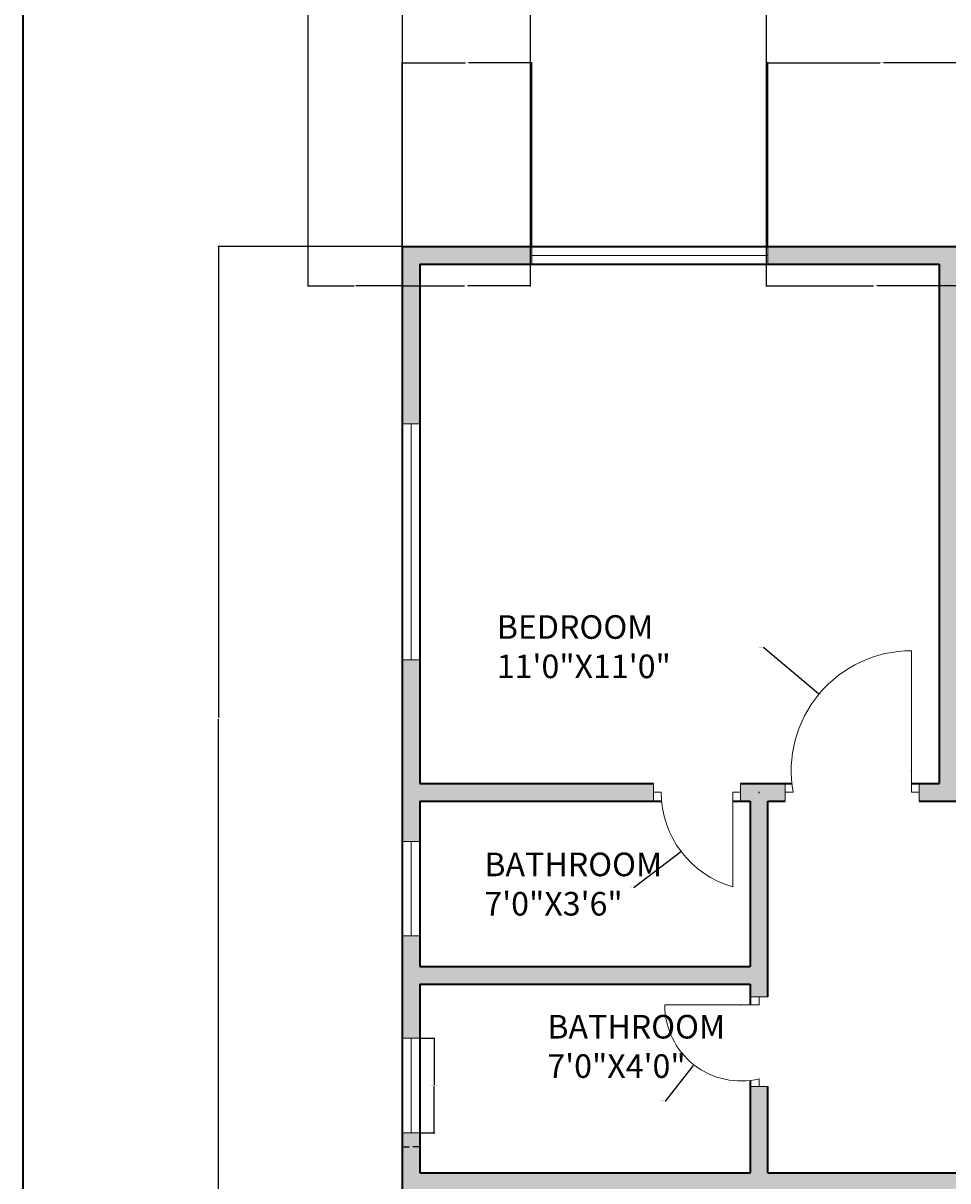
# Model space of a CAD drawing. Units: inches. Extents: x 2314 to 3223, y 1382 to 2735.
# Tile 8 of 14: x 2314 to 2549, y 2144 to 2439. Entities that reach past the tile are written whole.
import ezdxf

# ---------------------------------------------------------------- set-up
doc = ezdxf.new("R2010")
doc.units = ezdxf.units.IN
for name, color, linetype, lineweight in [('A-ANNO-DIMS', 2, 'Continuous', 18), ('A-ANNO-TTLB', 7, 'Continuous', 35), ('A-AREA-IDEN', 7, 'Continuous', 18), ('A-DOOR', 3, 'Continuous', 18), ('A-GLAZ', 4, 'Continuous', 18), ('A-WALL', 7, 'Continuous', 35)]:
    doc.layers.add(name, color=color, linetype=linetype, lineweight=lineweight)
doc.layers.add('A-WALL-PATT', color=251, linetype='Continuous', lineweight=13, true_color=0x636466)
doc.styles.get("Standard").update_dxf_attribs({"font": 'arial.ttf'})
doc.dimstyles.get("Standard").update_dxf_attribs({"dimtxt": 0.18, "dimasz": 0.18, "dimexe": 0.18, "dimexo": 0.0625, "dimgap": 0.09, "dimtad": 0, "dimtih": 1, "dimtoh": 1, "dimdec": 4, "dimzin": 0, "dimdsep": 46, "dimtxsty": 'Standard', "dimcen": 0.09, "dimadec": 0, "dimazin": 0, "dimtfac": 1, "dimtdec": 4, "dimtofl": 0, "dimtmove": 0, "dimatfit": 3, "dimfxl": 1, "dimtolj": 1, "dimtzin": 0, "dimarcsym": 0})

# ---------------------------------------------------------------- blocks, each defined once
blk = doc.blocks.new('WIN-PLAN-24')
for p, q in [((0, 24), (4.5, 24)), ((4.5, 24), (2.25, 24)), ((2.25, 24), (2.25, 0)), ((2.25, 0), (0, 0)), ((0, 0), (4.5, 0))]:
    blk.add_line(p, q)
blk = doc.blocks.new('WIN-PLAN-24-ALT')
for p, q in [((4.5, 24), (0, 24)), ((0, 24), (2.25, 24)), ((2.25, 24), (2.25, 0)), ((2.25, 0), (0, 0)), ((0, 0), (4.5, 0))]:
    blk.add_line(p, q)
blk = doc.blocks.new('WIN-PLAN-60')
for p, q in [((0, 4.5), (0, 0)), ((60, 2.25), (60, 4.5)), ((60, 4.5), (60, 0)), ((0, 0), (0, 2.25)), ((0, 2.25), (60, 2.25))]:
    blk.add_line(p, q)
blk = doc.blocks.new('*D17')
at = {"layer": 'A-ANNO-DIMS', "color": 0, "lineweight": -2, "transparency": 16777216}
for p, q in [((2414.96, 2180.5), (2418.67, 2180.5)), ((2418.49, 2180.32), (2418.49, 2168.69)), ((2418.49, 2156.68), (2418.49, 2168.32)), ((2414.96, 2156.5), (2418.67, 2156.5))]:
    blk.add_line(p, q, dxfattribs=at)
at = {"layer": 'A-ANNO-DIMS', "color": 0, "transparency": 16777216}
for points in [[(2418.46, 2180.32), (2418.52, 2180.32), (2418.49, 2180.5)], [(2418.46, 2156.68), (2418.52, 2156.68), (2418.49, 2156.5)]]:
    blk.add_solid(points, dxfattribs=at)
at = {"layer": 'Defpoints', "color": 0, "transparency": 16777216}
for p in [(2414.89, 2180.5), (2418.49, 2180.5), (2414.89, 2156.5)]:
    blk.add_point(p, dxfattribs=at)
at = {"layer": 'A-ANNO-DIMS', "color": 0, "transparency": 16777216, "insert": (2418.49, 2168.5), "char_height": 0.18, "attachment_point": 5}
blk.add_mtext('\\A1;WINDOW 24 TYP.', dxfattribs=at)
blk = doc.blocks.new('*D18')
at = {"layer": 'A-ANNO-DIMS', "color": 0, "lineweight": -2, "transparency": 16777216}
for p, q in [((2410.39, 2156.44), (2410.39, 2152.72)), ((2414.89, 2156.44), (2414.89, 2152.72)), ((2410.57, 2152.9), (2412.18, 2152.9)), ((2414.71, 2152.9), (2413.1, 2152.9))]:
    blk.add_line(p, q, dxfattribs=at)
at = {"layer": 'A-ANNO-DIMS', "color": 0, "transparency": 16777216}
for points in [[(2410.57, 2152.93), (2410.57, 2152.87), (2410.39, 2152.9)], [(2414.71, 2152.93), (2414.71, 2152.87), (2414.89, 2152.9)]]:
    blk.add_solid(points, dxfattribs=at)
at = {"layer": 'Defpoints', "color": 0, "transparency": 16777216}
for p in [(2410.39, 2156.5), (2414.89, 2156.5), (2414.89, 2152.9)]:
    blk.add_point(p, dxfattribs=at)
at = {"layer": 'A-ANNO-DIMS', "color": 0, "transparency": 16777216, "insert": (2412.64, 2152.9), "char_height": 0.18, "attachment_point": 5}
blk.add_mtext('\\A1;5 TYP.', dxfattribs=at)
blk = doc.blocks.new('*D34')
at = {"layer": 'A-ANNO-DIMS', "color": 0, "lineweight": -2, "transparency": 16777216}
for p, q in [((2410.33, 2381.78), (2363.51, 2381.78)), ((2363.69, 2381.6), (2363.69, 2262.02)), ((2363.69, 2142.06), (2363.69, 2261.65)), ((2410.33, 2141.88), (2363.51, 2141.88))]:
    blk.add_line(p, q, dxfattribs=at)
at = {"layer": 'A-ANNO-DIMS', "color": 0, "transparency": 16777216}
for points in [[(2363.66, 2381.6), (2363.72, 2381.6), (2363.69, 2381.78)], [(2363.66, 2142.06), (2363.72, 2142.06), (2363.69, 2141.88)]]:
    blk.add_solid(points, dxfattribs=at)
at = {"layer": 'Defpoints', "color": 0, "transparency": 16777216}
for p in [(2363.69, 2381.78), (2410.39, 2381.78), (2410.39, 2141.88)]:
    blk.add_point(p, dxfattribs=at)
at = {"layer": 'A-ANNO-DIMS', "color": 0, "transparency": 16777216, "insert": (2363.69, 2261.83), "char_height": 0.18, "attachment_point": 5}
blk.add_mtext('\\A1;239.9', dxfattribs=at)
blk = doc.blocks.new('*D40')
at = {"layer": 'A-ANNO-DIMS', "color": 0, "lineweight": -2, "transparency": 16777216}
for p, q in [((2410.39, 2381.85), (2410.39, 2428.66)), ((2410.57, 2428.48), (2426.47, 2428.48)), ((2443.15, 2428.48), (2427.25, 2428.48)), ((2443.33, 2381.85), (2443.33, 2428.66))]:
    blk.add_line(p, q, dxfattribs=at)
at = {"layer": 'A-ANNO-DIMS', "color": 0, "transparency": 16777216}
for points in [[(2410.57, 2428.51), (2410.57, 2428.45), (2410.39, 2428.48)], [(2443.15, 2428.51), (2443.15, 2428.45), (2443.33, 2428.48)]]:
    blk.add_solid(points, dxfattribs=at)
at = {"layer": 'Defpoints', "color": 0, "transparency": 16777216}
for p in [(2443.33, 2428.48), (2410.39, 2381.78), (2443.33, 2381.78)]:
    blk.add_point(p, dxfattribs=at)
at = {"layer": 'A-ANNO-DIMS', "color": 0, "transparency": 16777216, "insert": (2426.86, 2428.48), "char_height": 0.18, "attachment_point": 5}
blk.add_mtext('\\A1;32.94', dxfattribs=at)
blk = doc.blocks.new('*D41')
at = {"layer": 'A-ANNO-DIMS', "color": 0, "lineweight": -2, "transparency": 16777216}
for p, q in [((2503.33, 2381.85), (2503.33, 2428.66)), ((2503.51, 2428.48), (2531.95, 2428.48)), ((2561.18, 2428.48), (2532.74, 2428.48)), ((2561.36, 2381.85), (2561.36, 2428.66))]:
    blk.add_line(p, q, dxfattribs=at)
at = {"layer": 'A-ANNO-DIMS', "color": 0, "transparency": 16777216}
for points in [[(2503.51, 2428.51), (2503.51, 2428.45), (2503.33, 2428.48)], [(2561.18, 2428.51), (2561.18, 2428.45), (2561.36, 2428.48)]]:
    blk.add_solid(points, dxfattribs=at)
at = {"layer": 'Defpoints', "color": 0, "transparency": 16777216}
for p in [(2561.36, 2428.48), (2503.33, 2381.78), (2561.36, 2381.78)]:
    blk.add_point(p, dxfattribs=at)
at = {"layer": 'A-ANNO-DIMS', "color": 0, "transparency": 16777216, "insert": (2532.35, 2428.48), "char_height": 0.18, "attachment_point": 5}
blk.add_mtext('\\A1;58.03', dxfattribs=at)
blk = doc.blocks.new('*D51')
at = {"layer": 'A-ANNO-DIMS', "color": 0, "lineweight": -2, "transparency": 16777216}
for p, q in [((2386.39, 2586.62), (2386.39, 2371.63)), ((2410.39, 2578.28), (2410.39, 2371.63)), ((2386.57, 2371.81), (2398.17, 2371.81)), ((2410.21, 2371.81), (2398.61, 2371.81))]:
    blk.add_line(p, q, dxfattribs=at)
at = {"layer": 'A-ANNO-DIMS', "color": 0, "transparency": 16777216}
for points in [[(2386.57, 2371.84), (2386.57, 2371.78), (2386.39, 2371.81)], [(2410.21, 2371.84), (2410.21, 2371.78), (2410.39, 2371.81)]]:
    blk.add_solid(points, dxfattribs=at)
at = {"layer": 'Defpoints', "color": 0, "transparency": 16777216}
for p in [(2386.39, 2586.68), (2410.39, 2578.34), (2410.39, 2371.81)]:
    blk.add_point(p, dxfattribs=at)
at = {"layer": 'A-ANNO-DIMS', "color": 0, "transparency": 16777216, "insert": (2398.39, 2371.81), "char_height": 0.18, "attachment_point": 5}
blk.add_mtext('\\A1;24', dxfattribs=at)
blk = doc.blocks.new('*D52')
at = {"layer": 'A-ANNO-DIMS', "color": 0, "lineweight": -2, "transparency": 16777216}
for p, q in [((2442.93, 2502.62), (2442.93, 2371.63)), ((2410.39, 2466.62), (2410.39, 2371.63)), ((2410.57, 2371.81), (2426.27, 2371.81)), ((2442.75, 2371.81), (2427.06, 2371.81))]:
    blk.add_line(p, q, dxfattribs=at)
at = {"layer": 'A-ANNO-DIMS', "color": 0, "transparency": 16777216}
for points in [[(2410.57, 2371.84), (2410.57, 2371.78), (2410.39, 2371.81)], [(2442.75, 2371.84), (2442.75, 2371.78), (2442.93, 2371.81)]]:
    blk.add_solid(points, dxfattribs=at)
at = {"layer": 'Defpoints', "color": 0, "transparency": 16777216}
for p in [(2442.93, 2502.68), (2410.39, 2466.68), (2442.93, 2371.81)]:
    blk.add_point(p, dxfattribs=at)
at = {"layer": 'A-ANNO-DIMS', "color": 0, "transparency": 16777216, "insert": (2426.66, 2371.81), "char_height": 0.18, "attachment_point": 5}
blk.add_mtext('\\A1;32.54', dxfattribs=at)
blk = doc.blocks.new('*D53')
at = {"layer": 'A-ANNO-DIMS', "color": 0, "lineweight": -2, "transparency": 16777216}
for p, q in [((2502.93, 2502.62), (2502.93, 2371.63)), ((2558.38, 2502.62), (2558.38, 2371.63)), ((2503.11, 2371.81), (2530.26, 2371.81)), ((2558.2, 2371.81), (2531.05, 2371.81))]:
    blk.add_line(p, q, dxfattribs=at)
at = {"layer": 'A-ANNO-DIMS', "color": 0, "transparency": 16777216}
for points in [[(2503.11, 2371.84), (2503.11, 2371.78), (2502.93, 2371.81)], [(2558.2, 2371.84), (2558.2, 2371.78), (2558.38, 2371.81)]]:
    blk.add_solid(points, dxfattribs=at)
at = {"layer": 'Defpoints', "color": 0, "transparency": 16777216}
for p in [(2502.93, 2502.68), (2558.38, 2502.68), (2558.38, 2371.81)]:
    blk.add_point(p, dxfattribs=at)
at = {"layer": 'A-ANNO-DIMS', "color": 0, "transparency": 16777216, "insert": (2530.66, 2371.81), "char_height": 0.18, "attachment_point": 5}
blk.add_mtext('\\A1;55.45', dxfattribs=at)
blk = doc.blocks.new('*D67')
at = {"layer": 'A-ANNO-DIMS', "color": 0, "lineweight": -2, "transparency": 16777216}
for p, q in [((2502.17, 2279.83), (2502.35, 2279.83)), ((2502.35, 2279.83), (2516.28, 2268.18)), ((2539.79, 2248.46), (2539.97, 2248.46)), ((2539.88, 2248.37), (2539.88, 2248.55))]:
    blk.add_line(p, q, dxfattribs=at)
at = {"layer": 'A-ANNO-DIMS', "color": 0, "transparency": 16777216}
blk.add_solid([(2516.3, 2268.2), (2516.26, 2268.16), (2516.42, 2268.07)], dxfattribs=at)
at = {"layer": 'Defpoints', "color": 0, "transparency": 16777216}
for p in [(2516.42, 2268.07), (2539.88, 2248.46)]:
    blk.add_point(p, dxfattribs=at)
at = {"layer": 'A-ANNO-DIMS', "color": 0, "transparency": 16777216, "insert": (2501.69, 2279.83), "char_height": 0.18, "attachment_point": 5}
blk.add_mtext('\\A1;R30.57', dxfattribs=at)
blk = doc.blocks.new('*D82')
at = {"layer": 'A-ANNO-DIMS', "color": 0, "lineweight": -2, "transparency": 16777216}
for p, q in [((2501.1, 2243.03), (2501.28, 2243.03)), ((2501.19, 2242.94), (2501.19, 2243.12)), ((2469.38, 2218.95), (2481.17, 2227.87)), ((2469.2, 2218.95), (2469.38, 2218.95))]:
    blk.add_line(p, q, dxfattribs=at)
at = {"layer": 'A-ANNO-DIMS', "color": 0, "transparency": 16777216}
blk.add_solid([(2481.15, 2227.9), (2481.19, 2227.85), (2481.31, 2227.98)], dxfattribs=at)
at = {"layer": 'Defpoints', "color": 0, "transparency": 16777216}
for p in [(2501.19, 2243.03), (2481.31, 2227.98)]:
    blk.add_point(p, dxfattribs=at)
at = {"layer": 'A-ANNO-DIMS', "color": 0, "transparency": 16777216, "insert": (2468.65, 2218.95), "char_height": 0.18, "attachment_point": 5}
blk.add_mtext('\\A1;R24.935', dxfattribs=at)
blk = doc.blocks.new('*D89')
at = {"layer": 'A-ANNO-DIMS', "color": 0, "lineweight": -2, "transparency": 16777216}
for p, q in [((2496.41, 2189.01), (2496.59, 2189.01)), ((2496.5, 2188.92), (2496.5, 2189.1)), ((2477.41, 2164.62), (2484.46, 2173.62)), ((2477.23, 2164.62), (2477.41, 2164.62))]:
    blk.add_line(p, q, dxfattribs=at)
at = {"layer": 'A-ANNO-DIMS', "color": 0, "transparency": 16777216}
blk.add_solid([(2484.43, 2173.64), (2484.48, 2173.61), (2484.57, 2173.77)], dxfattribs=at)
at = {"layer": 'Defpoints', "color": 0, "transparency": 16777216}
for p in [(2496.5, 2189.01), (2484.57, 2173.77)]:
    blk.add_point(p, dxfattribs=at)
at = {"layer": 'A-ANNO-DIMS', "color": 0, "transparency": 16777216, "insert": (2476.68, 2164.62), "char_height": 0.18, "attachment_point": 5}
blk.add_mtext('\\A1;R19.356', dxfattribs=at)

msp = doc.modelspace()

# ---------------------------------------------------------------- hatches: boundary and pattern name
at = {"layer": 'A-WALL-PATT'}
h = msp.add_hatch(color=256, dxfattribs=at)
h.dxf.hatch_style = 1
h.paths.add_polyline_path([(2443.3302, 2379.5332), (2443.3302, 2381.7832), (2410.3927, 2381.7832), (2410.3927, 2336.7008), (2414.8927, 2336.7008), (2414.8927, 2377.2832), (2443.3302, 2377.2832)])
h.paths.add_polyline_path([(2561.3645, 2379.5332), (2561.3645, 2381.7832), (2503.3302, 2381.7832), (2503.3302, 2377.2832), (2546.8927, 2377.2832), (2546.8927, 2245.2832), (2541.8787, 2245.2832), (2541.8787, 2240.7832), (2551.3927, 2240.7832), (2551.3927, 2377.2832), (2561.3645, 2377.2832)])
h.paths.add_polyline_path([(2656.0607, 2381.7832), (2597.3645, 2381.7832), (2597.3645, 2377.2832), (2617.3927, 2377.2832), (2617.3927, 2257.2832), (2584.2532, 2257.2832), (2584.2532, 2252.7832), (2625.8528, 2252.7832), (2625.8528, 2255.0332), (2625.8528, 2257.2832), (2621.8927, 2257.2832), (2621.8927, 2377.2832), (2656.0607, 2377.2832), (2656.0607, 2379.5332)])
h.paths.add_polyline_path([(2807.3418, 2381.7832), (2716.0607, 2381.7832), (2716.0607, 2377.2832), (2765.8927, 2377.2832), (2765.8927, 2257.2832), (2661.6935, 2257.2832), (2661.6935, 2252.7832), (2765.8927, 2252.7832), (2765.8927, 2146.2832), (2760.9259, 2146.2832), (2760.9259, 2141.8832), (2775.7119, 2141.8832), (2775.7119, 2146.2832), (2770.3927, 2146.2832), (2770.3927, 2252.7832), (2877.684, 2252.7832), (2877.684, 2255.0332), (2877.684, 2257.2832), (2770.3927, 2257.2832), (2770.3927, 2377.2832), (2807.3418, 2377.2832), (2807.3418, 2379.5332)])
h.paths.add_polyline_path([(2937.2118, 2381.7832), (2867.3418, 2381.7832), (2867.3418, 2377.2832), (2914.3927, 2377.2832), (2914.3927, 2257.2832), (2908.4124, 2257.2832), (2908.4124, 2252.7832), (2960.6432, 2252.7832), (2960.6432, 2255.0332), (2960.6432, 2257.2832), (2918.8927, 2257.2832), (2918.8927, 2377.2832), (2937.2118, 2377.2832)])
h.paths.add_polyline_path([(3022.1601, 2381.7832), (2973.2118, 2381.7832), (2973.2118, 2379.5332), (2973.2118, 2377.2832), (2984.8927, 2377.2832), (2984.8927, 2257.2832), (2980.0601, 2257.2832), (2980.0601, 2252.7832), (2984.8927, 2252.7832), (2984.8927, 2240.7832), (2995.668, 2240.7832), (2995.668, 2243.0332), (2995.668, 2245.2832), (2989.3927, 2245.2832), (2989.3927, 2377.2832), (3022.1601, 2377.2832), (3022.1601, 2379.5332)])
h.paths.add_polyline_path([(3125.8927, 2381.7832), (3082.1601, 2381.7832), (3082.1601, 2377.2832), (3121.3927, 2377.2832), (3121.3927, 2334.7388), (3125.8927, 2334.7388)])
h.paths.add_polyline_path([(3125.8927, 2274.7388), (3121.3927, 2274.7388), (3121.3927, 2245.2832), (3066.4832, 2245.2832), (3066.4832, 2240.7832), (3121.3927, 2240.7832), (3121.3927, 2232.1868), (3125.8927, 2232.1868)])
h.paths.add_polyline_path([(3125.8927, 2208.1868), (3121.3927, 2208.1868), (3121.3927, 2198.7832), (3037.3927, 2198.7832), (3037.3927, 2240.7832), (3041.2694, 2240.7832), (3041.2694, 2243.0332), (3041.2694, 2245.2832), (3026.8205, 2245.2832), (3026.8205, 2240.7832), (3032.8927, 2240.7832), (3032.8927, 2190.4022), (3037.3927, 2190.4022), (3037.3927, 2194.2832), (3121.3927, 2194.2832), (3121.3927, 2182.1835), (3125.8927, 2182.1835)])
h.paths.add_polyline_path([(3125.8927, 2158.1835), (3121.3927, 2158.1835), (3121.3927, 2146.2832), (3037.3927, 2146.2832), (3037.3927, 2169.3726), (3035.1427, 2169.3726), (3032.8927, 2169.3726), (3032.8927, 2146.2832), (2812.7301, 2146.2832), (2812.7301, 2144.0832), (2812.7301, 2141.8832), (2818.3927, 2141.8832), (2818.3927, 1970.1316), (2822.8927, 1970.1316), (2822.8927, 1978.8832), (2903.9846, 1978.8832), (2903.9846, 1981.1332), (2903.9846, 1983.3832), (2822.8927, 1983.3832), (2822.8927, 2115.3832), (2851.7162, 2115.3832), (2851.7162, 2117.6332), (2851.7162, 2119.8832), (2822.8927, 2119.8832), (2822.8927, 2141.8832), (3125.8927, 2141.8832)])
h.paths.add_polyline_path([(3125.8927, 2119.8832), (3081.193, 2119.8832), (3081.193, 2115.3832), (3121.3927, 2115.3832), (3121.3927, 2071.8188), (3125.8927, 2071.8188)], flags=17)
h.paths.add_polyline_path([(2989.3927, 2115.3832), (3021.193, 2115.3832), (3021.193, 2117.6332), (3021.193, 2119.8832), (2979.123, 2119.8832), (2979.123, 2115.3832), (2984.8927, 2115.3832), (2984.8927, 2019.3832), (2981.9225, 2019.3832), (2981.9225, 2014.8832), (2984.8927, 2014.8832), (2984.8927, 1983.3832), (2984.8927, 1978.8832), (2989.3927, 1978.8832), (2989.3927, 1983.3832)], flags=17)
h.paths.add_polyline_path([(2947.3927, 2115.3832), (2955.123, 2115.3832), (2955.123, 2117.6332), (2955.123, 2119.8832), (2911.7162, 2119.8832), (2911.7162, 2115.3832), (2942.8927, 2115.3832), (2942.8927, 1983.3832), (2936.7017, 1983.3832), (2936.7017, 1978.8832), (2947.3927, 1978.8832), (2947.3927, 1983.3832), (2947.3927, 2014.8832), (2960.7167, 2014.8832), (2960.7167, 2017.1332), (2960.7167, 2019.3832), (2947.3927, 2019.3832)], flags=17)
h.paths.add_polyline_path([(3037.3927, 1978.8832), (3041.8276, 1978.8832), (3041.8276, 1981.1332), (3041.8276, 1983.3832), (3025.477, 1983.3832), (3025.477, 1978.8832), (3032.8927, 1978.8832), (3032.8927, 1927.1259), (3035.1427, 1927.1259), (3037.3927, 1927.1259)])
h.paths.add_polyline_path([(3125.8927, 2011.8188), (3123.6427, 2011.8188), (3121.3927, 2011.8188), (3121.3927, 1983.3832), (3065, 1983.3832), (3065, 1978.8832), (3121.3927, 1978.8832), (3121.3927, 1970.5932), (3125.8927, 1970.5932)], flags=17)
h.paths.add_polyline_path([(2994.2341, 1983.3832), (2989.3927, 1983.3832), (2989.3927, 1978.8832), (2994.2341, 1978.8832), (2994.2341, 1981.1332)], flags=16)
h.paths.add_polyline_path([(3125.8927, 1946.5932), (3121.3927, 1946.5932), (3121.3927, 1936.8832), (3037.3927, 1936.8832), (3037.3927, 1932.3832), (3121.3927, 1932.3832), (3121.3927, 1919.825), (3125.8927, 1919.825)])
h.paths.add_polyline_path([(3125.8927, 1883.825), (3121.3927, 1883.825), (3121.3927, 1866.3832), (3037.3927, 1866.3832), (3037.3927, 1899.0954), (3035.1427, 1899.0954), (3032.8927, 1899.0954), (3032.8927, 1866.3832), (2822.8927, 1866.3832), (2822.8927, 1938.7212), (2820.6427, 1938.7212), (2818.3927, 1938.7212), (2818.3927, 1786.9239), (2822.8927, 1786.9239), (2822.8927, 1861.8832), (3032.8927, 1861.8832), (3032.8927, 1825.1023), (3037.3927, 1825.1023), (3037.3927, 1861.8832), (3121.3927, 1861.8832), (3121.3927, 1844.6765), (3125.8927, 1844.6765)])
h.paths.add_polyline_path([(3125.8927, 1808.6765), (3121.3927, 1808.6765), (3121.3927, 1795.8832), (3037.3927, 1795.8832), (3037.3927, 1799.4755), (3032.8927, 1799.4755), (3032.8927, 1749.3832), (3026.5034, 1749.3832), (3026.5034, 1744.8832), (3032.8927, 1744.8832), (3034.9255, 1744.8832), (3043.1326, 1744.8832), (3043.1326, 1747.1332), (3043.1326, 1749.3832), (3037.3927, 1749.3832), (3037.3927, 1791.3832), (3121.3927, 1791.3832), (3121.3927, 1783.3103), (3125.8927, 1783.3103)])
h.paths.add_polyline_path([(3125.8927, 1759.3103), (3121.3927, 1759.3103), (3121.3927, 1749.3832), (3065.1845, 1749.3832), (3065.1845, 1744.8832), (3121.3927, 1744.8832), (3121.3927, 1709.3573), (3125.8927, 1709.3573)])
h.paths.add_polyline_path([(3125.8927, 1649.3573), (3121.3927, 1649.3573), (3121.3927, 1612.8832), (3095.116, 1612.8832), (3095.116, 1608.3832), (3125.8927, 1608.3832)])
h.paths.add_polyline_path([(3035.116, 1612.8832), (2993.8927, 1612.8832), (2993.8927, 1744.8832), (2998.7409, 1744.8832), (2998.7409, 1749.3832), (2989.3927, 1749.3832), (2989.3927, 1744.8832), (2989.3927, 1701.3832), (2972.8226, 1701.3832), (2972.8226, 1696.8832), (2989.3927, 1696.8832), (2989.3927, 1612.8832), (2978.2225, 1612.8832), (2978.2225, 1608.3832), (3035.116, 1608.3832), (3035.116, 1610.6332)])
h.paths.add_polyline_path([(2947.3927, 1696.8832), (2950.7566, 1696.8832), (2950.7566, 1699.1332), (2950.7566, 1701.3832), (2947.3927, 1701.3832), (2947.3927, 1744.8832), (2947.3927, 1749.3832), (2937.649, 1749.3832), (2937.649, 1744.8832), (2942.8927, 1744.8832), (2942.8927, 1612.8832), (2907.783, 1612.8832), (2907.783, 1608.3832), (2954.2225, 1608.3832), (2954.2225, 1610.6332), (2954.2225, 1612.8832), (2947.3927, 1612.8832)])
h.paths.add_polyline_path([(2822.8927, 1744.8832), (2905.3491, 1744.8832), (2905.3491, 1747.1332), (2905.3491, 1749.3832), (2822.8927, 1749.3832), (2822.8927, 1756.9185), (2818.3927, 1756.9185), (2818.3927, 1612.8832), (2818.3927, 1569.1205), (2722.3927, 1569.1205), (2722.3927, 1612.8832), (2722.3927, 1756.9185), (2717.8927, 1756.9185), (2717.8927, 1750.0143), (2633.6297, 1750.0143), (2633.6437, 1745.2665), (2717.8927, 1745.5143), (2717.8927, 1612.8832), (2689.8467, 1612.8832), (2689.8467, 1608.3832), (2717.8927, 1608.3832), (2717.8927, 1564.6205), (2722.3927, 1564.6205), (2822.8927, 1564.6205), (2822.8927, 1569.1205), (2822.8927, 1608.3832), (2847.783, 1608.3832), (2847.783, 1610.6332), (2847.783, 1612.8832), (2822.8927, 1612.8832)])
h.paths.add_polyline_path([(2629.8467, 1612.8832), (2597.8927, 1612.8832), (2597.8927, 1744.8832), (2597.8927, 1745.1613), (2601.5887, 1745.1721), (2601.5816, 1747.5932), (2601.5745, 1750.0143), (2593.3927, 1750.0143), (2593.3927, 1744.8832), (2593.3927, 1713.3832), (2589.7588, 1713.3832), (2589.7588, 1708.8832), (2593.3927, 1708.8832), (2593.3927, 1612.8832), (2582.3793, 1612.8832), (2582.3793, 1608.3832), (2629.8467, 1608.3832), (2629.8467, 1610.6332)])
h.paths.add_polyline_path([(2551.3927, 1708.8832), (2567.6776, 1708.8832), (2567.6776, 1711.1332), (2567.6776, 1713.3832), (2551.3927, 1713.3832), (2551.3927, 1744.8832), (2551.3927, 1750.0143), (2543.5657, 1750.0143), (2543.5657, 1747.5079), (2543.5657, 1745.0014), (2546.8927, 1745.0112), (2546.8927, 1744.8832), (2546.8927, 1612.8832), (2502.9339, 1612.8832), (2502.9339, 1608.3832), (2558.3793, 1608.3832), (2558.3793, 1610.6332), (2558.3793, 1612.8832), (2551.3927, 1612.8832)])
h.paths.add_polyline_path([(2414.8927, 1656.2547), (2410.3927, 1656.2547), (2410.3927, 1608.3832), (2442.9339, 1608.3832), (2442.9339, 1610.6332), (2442.9339, 1612.8832), (2414.8927, 1612.8832)])
h.paths.add_polyline_path([(2414.8927, 1744.8832), (2468.8906, 1744.8832), (2468.8906, 1747.1332), (2468.8906, 1749.3832), (2414.8927, 1749.3832), (2414.8927, 1757.7622), (2410.3927, 1757.7622), (2410.3927, 1716.2547), (2414.8927, 1716.2547)])
h.paths.add_polyline_path([(2414.8927, 1791.3832), (2498.8927, 1791.3832), (2498.8927, 1749.3832), (2492.9799, 1749.3832), (2492.9799, 1744.8832), (2498.8927, 1744.8832), (2503.3927, 1744.8832), (2508.0135, 1744.8968), (2508.0059, 1747.4556), (2507.9984, 1750.0143), (2503.3927, 1750.0143), (2503.3927, 1802.6362), (2501.1427, 1802.6362), (2498.8927, 1802.6362), (2498.8927, 1795.8832), (2414.8927, 1795.8832), (2414.8927, 1808.0943), (2410.3927, 1808.0943), (2410.3927, 1781.7622), (2414.8927, 1781.7622)])
h.paths.add_polyline_path([(2722.3927, 1937.589), (2720.1427, 1937.589), (2717.8927, 1937.589), (2717.8927, 1866.3832), (2503.3927, 1866.3832), (2503.3927, 1896.3484), (2498.8927, 1896.3484), (2498.8927, 1866.3832), (2414.8927, 1866.3832), (2414.8927, 1882.1496), (2410.3927, 1882.1496), (2410.3927, 1844.0943), (2414.8927, 1844.0943), (2414.8927, 1861.8832), (2498.8927, 1861.8832), (2498.8927, 1831.4783), (2501.1427, 1831.4783), (2503.3927, 1831.4783), (2503.3927, 1861.8832), (2717.8927, 1861.8832), (2717.8927, 1786.9239), (2722.3927, 1786.9239)])
h.paths.add_polyline_path([(2414.8927, 1932.3832), (2498.8927, 1932.3832), (2498.8927, 1924.7883), (2503.3927, 1924.7883), (2503.3927, 1978.8832), (2505.8599, 1978.8832), (2505.8599, 1981.1332), (2505.8599, 1983.3832), (2493.3697, 1983.3832), (2493.3697, 1978.8832), (2498.8927, 1978.8832), (2498.8927, 1936.8832), (2414.8927, 1936.8832), (2414.8927, 1943.2834), (2410.3927, 1943.2834), (2410.3927, 1918.1496), (2414.8927, 1918.1496)])
h.paths.add_polyline_path([(2414.8927, 2020.3133), (2412.6427, 2020.3133), (2410.3927, 2020.3133), (2410.3927, 1967.2834), (2414.8927, 1967.2834), (2414.8927, 1978.8832), (2468.8513, 1978.8832), (2468.8513, 1981.1332), (2468.8513, 1983.3832), (2414.8927, 1983.3832)])
h.paths.add_polyline_path([(2414.8927, 2115.3832), (2453.004, 2115.3832), (2453.004, 2117.6332), (2453.004, 2119.8832), (2410.3927, 2119.8832), (2410.3927, 2080.3133), (2414.8927, 2080.3133)], flags=17)
h.paths.add_polyline_path([(2559.0969, 2117.6332), (2559.0969, 2119.8832), (2513.004, 2119.8832), (2513.004, 2115.3832), (2546.8927, 2115.3832), (2546.8927, 1983.3832), (2542.7531, 1983.3832), (2542.7531, 1978.8832), (2551.3927, 1978.8832), (2551.3927, 2014.8832), (2570.3098, 2014.8832), (2570.3098, 2017.1332), (2570.3098, 2019.3832), (2551.3927, 2019.3832), (2551.3927, 2115.3832), (2559.0969, 2115.3832)], flags=17)
h.paths.add_polyline_path([(2628.5073, 2117.6332), (2628.5073, 2119.8832), (2583.0969, 2119.8832), (2583.0969, 2115.3832), (2593.3927, 2115.3832), (2593.3927, 2019.3832), (2590.2108, 2019.3832), (2590.2108, 2014.8832), (2593.3927, 2014.8832), (2593.3927, 1978.8832), (2601.5907, 1978.8832), (2601.5907, 1981.1332), (2601.5907, 1983.3832), (2597.8927, 1983.3832), (2597.8927, 2115.3832), (2628.5073, 2115.3832)], flags=17)
h.paths.add_polyline_path([(2722.3927, 2141.8832), (2726.9871, 2141.8832), (2726.9871, 2144.2705), (2726.9871, 2146.2832), (2503.3927, 2146.2832), (2503.3927, 2168.2161), (2501.1427, 2168.2161), (2498.8927, 2168.2161), (2498.8927, 2146.2832), (2414.8927, 2146.2832), (2414.8927, 2156.5041), (2410.3927, 2156.5041), (2410.3927, 2141.8832), (2717.8927, 2141.8832), (2717.8927, 2119.8832), (2688.5073, 2119.8832), (2688.5073, 2115.3832), (2717.8927, 2115.3832), (2717.8927, 1983.3832), (2633.2454, 1983.3832), (2633.2454, 1978.8832), (2717.8927, 1978.8832), (2717.8927, 1970.1316), (2720.1427, 1970.1316), (2722.3927, 1970.1316)])
h.paths.add_polyline_path([(2557.3704, 1462.9278), (2940.0934, 1462.9278), (2940.0934, 1512.3848), (2557.3704, 1512.3848)], flags=9)
h.paths.add_polyline_path([(2846.2527, 1703.1384), (2892.8612, 1703.1384), (2892.8612, 1725.5272), (2846.2527, 1725.5272)], flags=25)
h.paths.add_polyline_path([(2885.6102, 1812.1147), (2946.1505, 1812.1147), (2946.1505, 1834.5035), (2885.6102, 1834.5035)], flags=25)
h.paths.add_polyline_path([(2885.6102, 1884.183), (2946.1505, 1884.183), (2946.1505, 1906.5718), (2885.6102, 1906.5718)], flags=25)
h.paths.add_polyline_path([(3066.365, 1705.5431), (3112.9735, 1705.5431), (3112.9735, 1727.9319), (3066.365, 1727.9319)], flags=9)
h.paths.add_polyline_path([(3061.8255, 1887.7513), (3101.6154, 1887.7513), (3101.6154, 1910.1401), (3061.8255, 1910.1401)], flags=25)
h.paths.add_polyline_path([(3063.3679, 1816.2121), (3103.1578, 1816.2121), (3103.1578, 1838.6009), (3063.3679, 1838.6009)], flags=25)
h.paths.add_polyline_path([(3053.3743, 1768.416), (3107.1329, 1768.416), (3107.1329, 1790.8048), (3053.3743, 1790.8048)], flags=25)
h.paths.add_polyline_path([(3061.6068, 1943.822), (3115.3653, 1943.822), (3115.3653, 1966.2109), (3061.6068, 1966.2109)], flags=9)
h.paths.add_polyline_path([(2745.0978, 1763.6604), (2797.9354, 1763.6604), (2797.9354, 1776.0247), (2745.0978, 1776.0247)], flags=9)
h.paths.add_polyline_path([(2574.2135, 1819.2586), (2634.7538, 1819.2586), (2634.7538, 1841.6474), (2574.2135, 1841.6474)], flags=25)
h.paths.add_polyline_path([(2574.2135, 1891.3269), (2634.7538, 1891.3269), (2634.7538, 1913.7157), (2574.2135, 1913.7157)], flags=25)
h.paths.add_polyline_path([(2638.4466, 1702.43), (2685.0551, 1702.43), (2685.0551, 1724.8188), (2638.4466, 1724.8188)], flags=25)
h.paths.add_polyline_path([(2435.9715, 1697.1215), (2482.5799, 1697.1215), (2482.5799, 1719.5103), (2435.9715, 1719.5103)], flags=9)
h.paths.add_polyline_path([(2431.2046, 1893.7833), (2470.9945, 1893.7833), (2470.9945, 1916.1721), (2431.2046, 1916.1721)], flags=25)
h.paths.add_polyline_path([(2439.8144, 1817.2116), (2479.6043, 1817.2116), (2479.6043, 1839.6004), (2439.8144, 1839.6004)], flags=25)
h.paths.add_polyline_path([(2441.2607, 1753.0942), (2495.0192, 1753.0942), (2495.0192, 1775.483), (2441.2607, 1775.483)], flags=25)
h.paths.add_polyline_path([(2421.216, 1945.3109), (2474.9746, 1945.3109), (2474.9746, 1967.6997), (2421.216, 1967.6997)], flags=25)
h.paths.add_polyline_path([(2585.4464, 1627.5703), (2585.4464, 1679), (2563.0576, 1679), (2563.0576, 1627.5703)], flags=9)
h.paths.add_polyline_path([(2978.3497, 1618.7039), (2978.3497, 1670.1337), (2955.9609, 1670.1337), (2955.9609, 1618.7039)], flags=9)
h.paths.add_polyline_path([(2975.9502, 2041.7828), (2975.9502, 2093.2125), (2953.5614, 2093.2125), (2953.5614, 2041.7828)], flags=25)
h.paths.add_polyline_path([(2835.6537, 1989.2068), (2882.2621, 1989.2068), (2882.2621, 2011.5956), (2835.6537, 2011.5956)], flags=25)
h.paths.add_polyline_path([(2649.3769, 1997.5659), (2695.9853, 1997.5659), (2695.9853, 2019.9547), (2649.3769, 2019.9547)], flags=25)
h.paths.add_polyline_path([(2579.9087, 2040.3429), (2579.9087, 2091.7726), (2557.5198, 2091.7726), (2557.5198, 2040.3429)], flags=25)
h.paths.add_polyline_path([(2783.2404, 1883.1956), (2783.2404, 2067.1369), (2764.694, 2067.1369), (2764.694, 1883.1956)], flags=9)
h.paths.add_polyline_path([(3055.8435, 1993.5571), (3102.4519, 1993.5571), (3102.4519, 2015.9459), (3055.8435, 2015.9459)], flags=25)
h.paths.add_polyline_path([(2423.6009, 1984.6082), (2470.2094, 1984.6082), (2470.2094, 2006.997), (2423.6009, 2006.997)], flags=25)
h.paths.add_polyline_path([(2973.4115, 2123.1668), (3013.1319, 2123.1668), (3013.1319, 2135.531), (2973.4115, 2135.531)], flags=25)
h.paths.add_polyline_path([(2534.3846, 2124.6231), (2574.105, 2124.6231), (2574.105, 2136.9874), (2534.3846, 2136.9874)], flags=25)
h.paths.add_polyline_path([(2829.1368, 2188.1931), (2889.411, 2188.1931), (2889.411, 2210.5819), (2829.1368, 2210.5819)], flags=9)
h.paths.add_polyline_path([(2633.2547, 2185.0437), (2693.5289, 2185.0437), (2693.5289, 2207.4325), (2633.2547, 2207.4325)], flags=9)
h.paths.add_polyline_path([(2445.1812, 2167.0395), (2496.611, 2167.0395), (2496.611, 2189.4284), (2445.1812, 2189.4284)], flags=9)
h.paths.add_polyline_path([(2429.1678, 2194.5482), (2480.5975, 2194.5482), (2480.5975, 2216.937), (2429.1678, 2216.937)], flags=9)
h.paths.add_polyline_path([(3060.1138, 2158.1056), (3111.5436, 2158.1056), (3111.5436, 2180.4944), (3060.1138, 2180.4944)], flags=9)
h.paths.add_polyline_path([(3055.6824, 2201.2631), (3107.1122, 2201.2631), (3107.1122, 2223.652), (3055.6824, 2223.652)], flags=25)
h.paths.add_polyline_path([(3044.3482, 2257.7345), (3090.9567, 2257.7345), (3090.9567, 2280.1233), (3044.3482, 2280.1233)], flags=9)
h.paths.add_polyline_path([(2942.5437, 2306.9625), (2982.3336, 2306.9625), (2982.3336, 2329.3513), (2942.5437, 2329.3513)], flags=9)
h.paths.add_polyline_path([(2799.5865, 2259.1663), (2846.195, 2259.1663), (2846.195, 2281.5551), (2799.5865, 2281.5551)], flags=25)
h.paths.add_polyline_path([(2670.4998, 2261.1493), (2717.1082, 2261.1493), (2717.1082, 2283.5381), (2670.4998, 2283.5381)], flags=25)
h.paths.add_polyline_path([(2553.0333, 2302.7735), (2592.8232, 2302.7735), (2592.8232, 2325.1624), (2553.0333, 2325.1624)], flags=9)
h.paths.add_polyline_path([(2432.0288, 2268.6489), (2478.6372, 2268.6489), (2478.6372, 2291.0377), (2432.0288, 2291.0377)], flags=9)
h = msp.add_hatch(color=256, dxfattribs=at)
h.dxf.hatch_style = 1
h.paths.add_polyline_path([(2503.3927, 2240.7832), (2507.7952, 2240.7832), (2507.7952, 2245.2832), (2496.4262, 2245.2832), (2496.4262, 2243.0332), (2496.4262, 2240.7832), (2498.8927, 2240.7832), (2498.8927, 2198.7832), (2414.8927, 2198.7832), (2414.8927, 2206.5718), (2410.3927, 2206.5718), (2410.3927, 2180.5041), (2412.6427, 2180.5041), (2414.8927, 2180.5041), (2414.8927, 2194.2832), (2498.8927, 2194.2832), (2498.8927, 2191.0069), (2503.3927, 2191.0069)])
h.paths.add_polyline_path([(2414.8927, 2276.7008), (2410.3927, 2276.7008), (2410.3927, 2230.5718), (2414.8927, 2230.5718), (2414.8927, 2240.7832), (2474.2564, 2240.7832), (2474.2564, 2243.0332), (2474.2564, 2245.2832), (2414.8927, 2245.2832)])
h.paths.add_polyline_path([(2557.3704, 1462.9278), (2940.0934, 1462.9278), (2940.0934, 1512.3848), (2557.3704, 1512.3848)], flags=9)
h.paths.add_polyline_path([(2846.2527, 1703.1384), (2892.8612, 1703.1384), (2892.8612, 1725.5272), (2846.2527, 1725.5272)], flags=9)
h.paths.add_polyline_path([(2885.6102, 1812.1147), (2946.1505, 1812.1147), (2946.1505, 1834.5035), (2885.6102, 1834.5035)], flags=9)
h.paths.add_polyline_path([(2885.6102, 1884.183), (2946.1505, 1884.183), (2946.1505, 1906.5718), (2885.6102, 1906.5718)], flags=9)
h.paths.add_polyline_path([(3066.365, 1705.5431), (3112.9735, 1705.5431), (3112.9735, 1727.9319), (3066.365, 1727.9319)], flags=9)
h.paths.add_polyline_path([(3061.8255, 1887.7513), (3101.6154, 1887.7513), (3101.6154, 1910.1401), (3061.8255, 1910.1401)], flags=9)
h.paths.add_polyline_path([(3063.3679, 1816.2121), (3103.1578, 1816.2121), (3103.1578, 1838.6009), (3063.3679, 1838.6009)], flags=9)
h.paths.add_polyline_path([(3053.3743, 1768.416), (3107.1329, 1768.416), (3107.1329, 1790.8048), (3053.3743, 1790.8048)], flags=9)
h.paths.add_polyline_path([(3061.6068, 1943.822), (3115.3653, 1943.822), (3115.3653, 1966.2109), (3061.6068, 1966.2109)], flags=9)
h.paths.add_polyline_path([(2745.0978, 1763.6604), (2797.9354, 1763.6604), (2797.9354, 1776.0247), (2745.0978, 1776.0247)], flags=9)
h.paths.add_polyline_path([(2574.2135, 1819.2586), (2634.7538, 1819.2586), (2634.7538, 1841.6474), (2574.2135, 1841.6474)], flags=9)
h.paths.add_polyline_path([(2574.2135, 1891.3269), (2634.7538, 1891.3269), (2634.7538, 1913.7157), (2574.2135, 1913.7157)], flags=9)
h.paths.add_polyline_path([(2638.4466, 1702.43), (2685.0551, 1702.43), (2685.0551, 1724.8188), (2638.4466, 1724.8188)], flags=9)
h.paths.add_polyline_path([(2435.9715, 1697.1215), (2482.5799, 1697.1215), (2482.5799, 1719.5103), (2435.9715, 1719.5103)], flags=9)
h.paths.add_polyline_path([(2431.2046, 1893.7833), (2470.9945, 1893.7833), (2470.9945, 1916.1721), (2431.2046, 1916.1721)], flags=9)
h.paths.add_polyline_path([(2439.8144, 1817.2116), (2479.6043, 1817.2116), (2479.6043, 1839.6004), (2439.8144, 1839.6004)], flags=9)
h.paths.add_polyline_path([(2441.2607, 1753.0942), (2495.0192, 1753.0942), (2495.0192, 1775.483), (2441.2607, 1775.483)], flags=9)
h.paths.add_polyline_path([(2421.216, 1945.3109), (2474.9746, 1945.3109), (2474.9746, 1967.6997), (2421.216, 1967.6997)], flags=9)
h.paths.add_polyline_path([(2585.4464, 1627.5703), (2585.4464, 1679), (2563.0576, 1679), (2563.0576, 1627.5703)], flags=9)
h.paths.add_polyline_path([(2978.3497, 1618.7039), (2978.3497, 1670.1337), (2955.9609, 1670.1337), (2955.9609, 1618.7039)], flags=9)
h.paths.add_polyline_path([(2975.9502, 2041.7828), (2975.9502, 2093.2125), (2953.5614, 2093.2125), (2953.5614, 2041.7828)], flags=9)
h.paths.add_polyline_path([(2835.6537, 1989.2068), (2882.2621, 1989.2068), (2882.2621, 2011.5956), (2835.6537, 2011.5956)], flags=9)
h.paths.add_polyline_path([(2649.3769, 1997.5659), (2695.9853, 1997.5659), (2695.9853, 2019.9547), (2649.3769, 2019.9547)], flags=9)
h.paths.add_polyline_path([(2579.9087, 2040.3429), (2579.9087, 2091.7726), (2557.5198, 2091.7726), (2557.5198, 2040.3429)], flags=9)
h.paths.add_polyline_path([(2783.2404, 1883.1956), (2783.2404, 2067.1369), (2764.694, 2067.1369), (2764.694, 1883.1956)], flags=9)
h.paths.add_polyline_path([(3055.8435, 1993.5571), (3102.4519, 1993.5571), (3102.4519, 2015.9459), (3055.8435, 2015.9459)], flags=9)
h.paths.add_polyline_path([(2423.6009, 1984.6082), (2470.2094, 1984.6082), (2470.2094, 2006.997), (2423.6009, 2006.997)], flags=9)
h.paths.add_polyline_path([(2973.4115, 2123.1668), (3013.1319, 2123.1668), (3013.1319, 2135.531), (2973.4115, 2135.531)], flags=9)
h.paths.add_polyline_path([(2534.3846, 2124.6231), (2574.105, 2124.6231), (2574.105, 2136.9874), (2534.3846, 2136.9874)], flags=9)
h.paths.add_polyline_path([(2829.1368, 2188.1931), (2889.411, 2188.1931), (2889.411, 2210.5819), (2829.1368, 2210.5819)], flags=9)
h.paths.add_polyline_path([(2633.2547, 2185.0437), (2693.5289, 2185.0437), (2693.5289, 2207.4325), (2633.2547, 2207.4325)], flags=9)
h.paths.add_polyline_path([(2445.1812, 2167.0395), (2496.611, 2167.0395), (2496.611, 2189.4284), (2445.1812, 2189.4284)], flags=9)
h.paths.add_polyline_path([(2429.1678, 2208.3022), (2480.5975, 2208.3022), (2480.5975, 2230.691), (2429.1678, 2230.691)], flags=25)
h.paths.add_polyline_path([(3060.1138, 2158.1056), (3111.5436, 2158.1056), (3111.5436, 2180.4944), (3060.1138, 2180.4944)], flags=9)
h.paths.add_polyline_path([(3055.6824, 2201.2631), (3107.1122, 2201.2631), (3107.1122, 2223.652), (3055.6824, 2223.652)], flags=9)
h.paths.add_polyline_path([(3044.3482, 2257.7345), (3090.9567, 2257.7345), (3090.9567, 2280.1233), (3044.3482, 2280.1233)], flags=9)
h.paths.add_polyline_path([(2942.5437, 2306.9625), (2982.3336, 2306.9625), (2982.3336, 2329.3513), (2942.5437, 2329.3513)], flags=9)
h.paths.add_polyline_path([(2799.5865, 2259.1663), (2846.195, 2259.1663), (2846.195, 2281.5551), (2799.5865, 2281.5551)], flags=9)
h.paths.add_polyline_path([(2670.4998, 2261.1493), (2717.1082, 2261.1493), (2717.1082, 2283.5381), (2670.4998, 2283.5381)], flags=9)
h.paths.add_polyline_path([(2553.0333, 2302.7735), (2592.8232, 2302.7735), (2592.8232, 2325.1624), (2553.0333, 2325.1624)], flags=9)
h.paths.add_polyline_path([(2432.0288, 2268.6489), (2478.6372, 2268.6489), (2478.6372, 2291.0377), (2432.0288, 2291.0377)], flags=9)

# ---------------------------------------------------------------- linework, layer by layer
at = {"layer": 'A-ANNO-TTLB'}
msp.add_lwpolyline([(2314.008, 2735.417), (3222.6676, 2735.417), (3222.6676, 1382.0876), (2314.008, 1382.0876)], close=True, dxfattribs=at)
at = {"layer": 'A-DOOR'}
for p, q in [((2539.8787, 2243.0332), (2539.8787, 2279.0332)), ((2474.2564, 2245.2832), (2474.2564, 2240.7832)), ((2474.2564, 2240.7832), (2474.2564, 2243.0332)), ((2474.2564, 2243.0332), (2476.2564, 2243.0332)), ((2496.4262, 2243.0332), (2494.4262, 2243.0332)), ((2494.4262, 2243.0332), (2494.4262, 2219.0332)), ((2496.4262, 2240.7832), (2496.4262, 2245.2832)), ((2496.4262, 2245.2832), (2496.4262, 2243.0332)), ((2507.7952, 2245.2832), (2507.7952, 2240.7832)), ((2507.7952, 2243.0332), (2509.7952, 2243.0332)), ((2541.8787, 2243.0332), (2539.8787, 2243.0332)), ((2541.8787, 2245.2832), (2541.8787, 2240.7832)), ((2541.8787, 2240.7832), (2541.8787, 2243.0332)), ((2498.8927, 2191.0069), (2503.3927, 2191.0069)), ((2503.3927, 2191.0069), (2501.1427, 2191.0069)), ((2501.1427, 2191.0069), (2501.1427, 2189.0069)), ((2501.1427, 2189.0069), (2477.1427, 2189.0069)), ((2501.1427, 2168.2161), (2501.1427, 2170.2161)), ((2498.8927, 2168.2161), (2503.3927, 2168.2161)), ((2503.3927, 2168.2161), (2501.1427, 2168.2161))]:
    msp.add_line(p, q, dxfattribs=at)
for centre, radius, start, end in [((2539.8787, 2248.4636), 30.5697, 90, 190.232216), ((2501.1917, 2243.0332), 24.9354, 180, 254.25702), ((2496.4988, 2189.0069), 19.3562, 180, 283.881567)]:
    msp.add_arc(centre, radius, start, end, dxfattribs=at)
at = {"layer": 'A-WALL'}
for p, q in [((2410.3927, 2381.7832), (3125.8927, 2381.7832)), ((2410.3927, 2381.7832), (2410.3927, 2141.8832)), ((2414.8927, 2377.2832), (2546.8927, 2377.2832)), ((2414.8927, 2377.2832), (2414.8927, 2245.2832)), ((2546.8927, 2377.2832), (2546.8927, 2245.2832)), ((2414.8927, 2245.2832), (2474.2564, 2245.2832)), ((2496.4262, 2245.2832), (2509.4749, 2245.2832)), ((2539.8787, 2245.2832), (2546.8927, 2245.2832)), ((2414.8927, 2240.7832), (2476.3581, 2240.7832)), ((2414.8927, 2240.7832), (2476.3581, 2240.7832)), ((2414.8927, 2240.7832), (2414.8927, 2198.7832)), ((2494.4262, 2240.7832), (2498.8927, 2240.7832)), ((2494.4262, 2240.7832), (2498.8927, 2240.7832)), ((2498.8927, 2240.7832), (2498.8927, 2198.7832)), ((2503.3927, 2240.7832), (2507.7952, 2240.7832)), ((2503.3927, 2191.0069), (2503.3927, 2240.7832)), ((2541.8787, 2240.7832), (2551.3927, 2240.7832)), ((2414.8927, 2198.7832), (2498.8927, 2198.7832)), ((2414.8927, 2194.2832), (2498.8927, 2194.2832)), ((2414.8927, 2194.2832), (2414.8927, 2146.2832)), ((2498.8927, 2194.2832), (2498.8927, 2189.0069)), ((2498.8927, 2169.7993), (2498.8927, 2146.2832)), ((2503.3927, 2146.2832), (2503.3927, 2168.2161)), ((2414.8927, 2146.2832), (2498.8927, 2146.2832)), ((2503.3927, 2146.2832), (2728.6937, 2146.2832))]:
    msp.add_line(p, q, dxfattribs=at)

# ---------------------------------------------------------------- block references
at = {"layer": 'A-GLAZ', "rotation": 180}
msp.add_blockref('WIN-PLAN-60', (2503.3302, 2381.7832), dxfattribs=at)
at = {"layer": 'A-GLAZ', "extrusion": (0, 0, -1), "zscale": -1, "rotation": 90}
msp.add_blockref('WIN-PLAN-60', (-2410.3927, 2276.7008), dxfattribs=at)
at = {"layer": 'A-GLAZ'}
for name, p in [('WIN-PLAN-24', (2410.3927, 2206.5718)), ('WIN-PLAN-24-ALT', (2410.3927, 2156.5041))]:
    msp.add_blockref(name, p, dxfattribs=at)

# ---------------------------------------------------------------- texts
at = {"layer": 'A-AREA-IDEN', "char_height": 6, "attachment_point": 1}
for s, width, insert in [('BEDROOM\\P11\'0"X11\'0"', 116.951221, (2434.4415, 2288.0561)), ('BATHROOM\\P7\'0"X3\'6"', 110.597382, (2431.2817, 2227.7095)), ('BATHROOM\\P7\'0"X4\'0"', 110.597382, (2447.2951, 2186.4468))]:
    msp.add_mtext_dynamic_manual_height_columns(s, width=width, gutter_width=12.5, heights=[0], dxfattribs=dict(at, insert=insert))

# ---------------------------------------------------------------- dimensions: what is measured, and where the dimension line sits
at = {"layer": 'A-ANNO-DIMS'}
for base, p1, p2, override, picture, middle in [((2410.3927, 2371.8121), (2386.3927, 2586.6793), (2410.3927, 2578.3383), {"dimdec": 0, "dimlfac": 1, "dimrnd": 0, "dimzin": 0, "dimdsep": 46, "dimlunit": 2}, '*D51', (2398.3927, 2371.8121)), ((2442.9339, 2371.8121), (2410.3927, 2466.6793), (2442.9339, 2502.6793), {"dimdec": 2, "dimlfac": 1, "dimrnd": 0, "dimzin": 0, "dimdsep": 46, "dimlunit": 2}, '*D52', (2426.6633, 2371.8121)), ((2558.3793, 2371.8121), (2502.9339, 2502.6793), (2558.3793, 2502.6793), {"dimdec": 2, "dimlfac": 1, "dimrnd": 0, "dimzin": 0, "dimdsep": 46, "dimlunit": 2}, '*D53', (2530.6566, 2371.8121)), ((2443.3302, 2428.4832), (2410.3927, 2381.7832), (2443.3302, 2381.7832), {"dimdec": 2, "dimlfac": 1, "dimrnd": 0, "dimzin": 0, "dimdsep": 46, "dimlunit": 2}, '*D40', (2426.8614, 2428.4832)), ((2561.3645, 2428.4832), (2503.3302, 2381.7832), (2561.3645, 2381.7832), {"dimdec": 2, "dimlfac": 1, "dimrnd": 0, "dimzin": 0, "dimdsep": 46, "dimlunit": 2}, '*D41', (2532.3474, 2428.4832))]:
    dim = msp.add_linear_dim(base=base, p1=p1, p2=p2, dimstyle='Standard', override=override, dxfattribs=at)
    dim.commit()
    dim.dimension.update_dxf_attribs({"geometry": picture, "text_midpoint": middle})
dim = msp.add_linear_dim(base=(2363.6927, 2381.7832), p1=(2410.3927, 2141.8832), p2=(2410.3927, 2381.7832), angle=90, dimstyle='Standard', override={"dimdec": 1, "dimlfac": 1, "dimrnd": 0, "dimzin": 0, "dimdsep": 46, "dimlunit": 2}, dxfattribs=at)
dim.commit()
dim.dimension.update_dxf_attribs({"geometry": '*D34', "text_midpoint": (2363.6927, 2261.8332)})
for center, mpoint, override, picture, middle in [((2539.8787, 2248.4636), (2516.4212, 2268.0659), {"dimdec": 2, "dimlfac": 1, "dimrnd": 0, "dimzin": 0, "dimdsep": 46, "dimlunit": 2}, '*D67', (2501.6868, 2279.8272)), ((2501.1917, 2243.0332), (2481.3112, 2227.9821), {"dimdec": 3, "dimlfac": 1, "dimrnd": 0, "dimzin": 0, "dimdsep": 46, "dimlunit": 2}, '*D82', (2468.6524, 2218.9515)), ((2496.4988, 2189.0069), (2484.5663, 2173.7663), {"dimdec": 3, "dimlfac": 1, "dimrnd": 0, "dimzin": 0, "dimdsep": 46, "dimlunit": 2}, '*D89', (2476.677, 2164.622))]:
    dim = msp.add_radius_dim(center=center, mpoint=mpoint, dimstyle='Standard', override=override, dxfattribs=at)
    dim.commit()
    dim.dimension.update_dxf_attribs({"geometry": picture, "text_midpoint": middle, "dimtype": 164})
dim = msp.add_linear_dim(base=(2418.4927, 2180.5041), p1=(2414.8927, 2156.5041), p2=(2414.8927, 2180.5041), angle=90, text='WINDOW <> TYP.', dimstyle='Standard', override={"dimdec": 0, "dimlfac": 1, "dimrnd": 0, "dimzin": 0, "dimdsep": 46, "dimlunit": 2}, dxfattribs=at)
dim.commit()
dim.dimension.update_dxf_attribs({"geometry": '*D17', "text_midpoint": (2418.4927, 2168.5041)})
dim = msp.add_linear_dim(base=(2414.8926767707, 2152.9040667736), p1=(2410.3926767707, 2156.5040667736), p2=(2414.8926767707, 2156.5040667736), text='<> TYP.', dimstyle='Standard', override={"dimdec": 0, "dimlfac": 1, "dimrnd": 0, "dimzin": 0, "dimdsep": 46, "dimlunit": 2}, dxfattribs=at)
dim.commit()
dim.dimension.update_dxf_attribs({"geometry": '*D18', "text_midpoint": (2412.6426767707, 2152.9040667736)})

doc.saveas('drawing.dxf')
